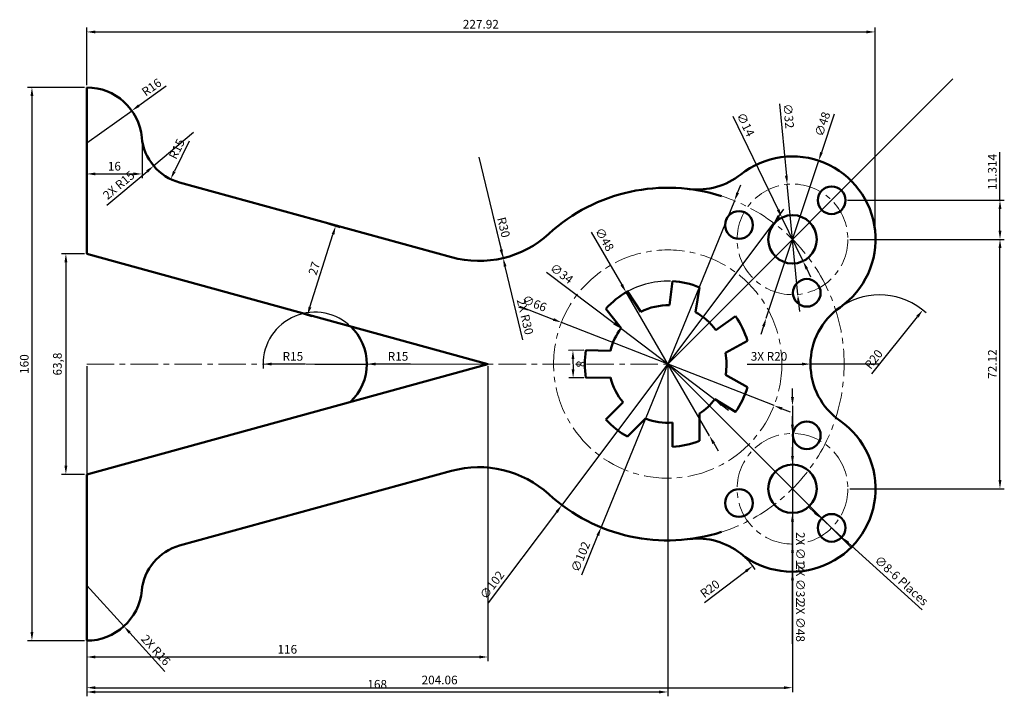
# Model space of a CAD drawing. Units: millimetres. Extents: x 1894 to 2178, y 716 to 912.
import ezdxf

# ---------------------------------------------------------------- set-up
doc = ezdxf.new("R2010")
doc.units = ezdxf.units.MM
doc.linetypes.add('CENTER', pattern=[50.8, 31.75, -6.35, 6.35, -6.35])
for name, color, linetype, lineweight in [('M-CNTR', 4, 'CENTER', 18), ('M-CONS', 8, 'Continuous', 13), ('M-DIMS', 2, 'Continuous', 25), ('M-OUTL', 7, 'Continuous', 50)]:
    doc.layers.add(name, color=color, linetype=linetype, lineweight=lineweight)
doc.styles.get("Standard").update_dxf_attribs({"font": 'arial.ttf'})
doc.dimstyles.new('ISO-25', dxfattribs={"dimtxt": 2.5, "dimasz": 2.5, "dimexe": 1.25, "dimexo": 0.625, "dimtad": 1, "dimtxsty": 'Standard', "dimcen": 2.5, "dimadec": 0, "dimazin": 0, "dimtfac": 1, "dimtmove": 0, "dimatfit": 3, "dimfxl": 1, "dimarcsym": 0})

# ---------------------------------------------------------------- blocks, each defined once
blk = doc.blocks.new('*U1')
blk.add_circle((0, 0), 4)
blk = doc.blocks.new('*U2')
at = {"layer": 'M-OUTL', "color": 0, "linetype": 'ByBlock', "lineweight": -2, "transparency": 16777216}
blk.add_blockref('*U1', (2128.28, 859.35), dxfattribs=at)
for p, rotation in [((2101.51, 852.18), 120), ((2121.11, 832.58), 240)]:
    blk.add_blockref('*U1', p, dxfattribs=dict(at, rotation=rotation))
blk = doc.blocks.new('*U3')
blk.add_circle((0, 0), 4)
blk = doc.blocks.new('*U4')
at = {"layer": 'M-OUTL', "color": 0, "linetype": 'ByBlock', "lineweight": -2, "transparency": 16777216}
for p, rotation in [((2121.11, 791.37), 120), ((2101.51, 771.77), 239.9999999999999)]:
    blk.add_blockref('*U3', p, dxfattribs=dict(at, rotation=rotation))
blk.add_blockref('*U3', (2128.28, 764.6), dxfattribs=at)
blk = doc.blocks.new('*D5')
at = {"layer": 'Defpoints', "color": 0, "transparency": 16777216}
for p in [(1912.93, 891.97), (1897.08, 731.97), (1912.91, 731.97)]:
    blk.add_point(p, dxfattribs=at)
at = {"layer": 'M-DIMS', "color": 0, "lineweight": -2, "transparency": 16777216}
for p, q in [((1912.3, 891.97), (1895.83, 891.97)), ((1897.08, 889.47), (1897.08, 734.47)), ((1912.28, 731.97), (1895.83, 731.97))]:
    blk.add_line(p, q, dxfattribs=at)
at = {"layer": 'M-DIMS', "color": 0, "transparency": 16777216}
for points in [[(1896.66, 889.47), (1897.5, 889.47), (1897.08, 891.97)], [(1896.66, 734.47), (1897.5, 734.47), (1897.08, 731.97)]]:
    blk.add_solid(points, dxfattribs=at)
at = {"layer": 'M-DIMS', "color": 0, "transparency": 16777216, "insert": (1895.18, 811.97), "char_height": 2.5, "attachment_point": 5, "rotation": 90}
blk.add_mtext('160', dxfattribs=at)
blk = doc.blocks.new('*D6')
at = {"layer": 'Defpoints', "color": 0, "transparency": 16777216}
for p in [(1912.91, 843.87), (1906.89, 780.07), (1912.91, 780.07)]:
    blk.add_point(p, dxfattribs=at)
at = {"layer": 'M-DIMS', "color": 0, "lineweight": -2, "transparency": 16777216}
for p, q in [((1912.28, 843.87), (1905.64, 843.87)), ((1906.89, 841.37), (1906.89, 782.57)), ((1912.28, 780.07), (1905.64, 780.07))]:
    blk.add_line(p, q, dxfattribs=at)
at = {"layer": 'M-DIMS', "color": 0, "transparency": 16777216}
for points in [[(1906.48, 841.37), (1907.31, 841.37), (1906.89, 843.87)], [(1906.48, 782.57), (1907.31, 782.57), (1906.89, 780.07)]]:
    blk.add_solid(points, dxfattribs=at)
at = {"layer": 'M-DIMS', "color": 0, "transparency": 16777216, "insert": (1904.76, 811.97), "char_height": 2.5, "attachment_point": 5, "rotation": 90}
blk.add_mtext('63,8', dxfattribs=at)
blk = doc.blocks.new('*D7')
at = {"layer": 'Defpoints', "color": 0, "transparency": 16777216}
for p in [(1912.91, 875.97), (1928.91, 875.97), (1928.91, 866.96)]:
    blk.add_point(p, dxfattribs=at)
at = {"layer": 'M-DIMS', "color": 0, "lineweight": -2, "transparency": 16777216}
for p, q in [((1912.91, 875.35), (1912.91, 865.71)), ((1928.91, 875.35), (1928.91, 865.71)), ((1915.41, 866.96), (1926.41, 866.96))]:
    blk.add_line(p, q, dxfattribs=at)
at = {"layer": 'M-DIMS', "color": 0, "transparency": 16777216}
for points in [[(1915.41, 867.38), (1915.41, 866.55), (1912.91, 866.96)], [(1926.41, 867.38), (1926.41, 866.55), (1928.91, 866.96)]]:
    blk.add_solid(points, dxfattribs=at)
at = {"layer": 'M-DIMS', "color": 0, "transparency": 16777216, "insert": (1920.91, 868.87), "char_height": 2.5, "attachment_point": 5}
blk.add_mtext('16', dxfattribs=at)
blk = doc.blocks.new('*D8')
at = {"layer": 'Defpoints', "color": 0, "transparency": 16777216}
for p in [(1979.07, 853.68), (1984.88, 851.84), (1970.91, 827.92)]:
    blk.add_point(p, dxfattribs=at)
at = {"layer": 'M-DIMS', "color": 0, "lineweight": -2, "transparency": 16777216}
for p, q in [((1979.67, 853.49), (1986.07, 851.46)), ((1977.47, 828.47), (1984.12, 849.46)), ((1971.5, 827.73), (1977.9, 825.71))]:
    blk.add_line(p, q, dxfattribs=at)
at = {"layer": 'M-DIMS', "color": 0, "transparency": 16777216}
for points in [[(1983.72, 849.58), (1984.52, 849.33), (1984.88, 851.84)], [(1977.07, 828.59), (1977.87, 828.34), (1976.71, 826.08)]]:
    blk.add_solid(points, dxfattribs=at)
at = {"layer": 'M-DIMS', "color": 0, "transparency": 16777216, "insert": (1979, 839.53), "char_height": 2.5, "attachment_point": 5, "rotation": 72.4174}
blk.add_mtext('27', dxfattribs=at)
blk = doc.blocks.new('*D9')
at = {"layer": 'Defpoints', "color": 0, "transparency": 16777216}
for p in [(1912.91, 811.97), (2028.91, 811.97), (2028.91, 727.25)]:
    blk.add_point(p, dxfattribs=at)
at = {"layer": 'M-DIMS', "color": 0, "lineweight": -2, "transparency": 16777216}
for p, q in [((1912.91, 811.35), (1912.91, 726)), ((2028.91, 811.35), (2028.91, 726)), ((1915.41, 727.25), (2026.41, 727.25))]:
    blk.add_line(p, q, dxfattribs=at)
at = {"layer": 'M-DIMS', "color": 0, "transparency": 16777216}
for points in [[(1915.41, 727.66), (1915.41, 726.83), (1912.91, 727.25)], [(2026.41, 727.66), (2026.41, 726.83), (2028.91, 727.25)]]:
    blk.add_solid(points, dxfattribs=at)
at = {"layer": 'M-DIMS', "color": 0, "transparency": 16777216, "insert": (1970.91, 729.15), "char_height": 2.5, "attachment_point": 5}
blk.add_mtext('116', dxfattribs=at)
blk = doc.blocks.new('*D10')
at = {"layer": 'Defpoints', "color": 0, "transparency": 16777216}
for p in [(2080.91, 811.97), (1912.91, 731.97), (2080.91, 717.13)]:
    blk.add_point(p, dxfattribs=at)
at = {"layer": 'M-DIMS', "color": 0, "lineweight": -2, "transparency": 16777216}
for p, q in [((2080.91, 811.35), (2080.91, 715.88)), ((1912.91, 731.35), (1912.91, 715.88)), ((1915.41, 717.13), (2078.41, 717.13))]:
    blk.add_line(p, q, dxfattribs=at)
at = {"layer": 'M-DIMS', "color": 0, "transparency": 16777216}
for points in [[(1915.41, 717.54), (1915.41, 716.71), (1912.91, 717.13)], [(2078.41, 717.54), (2078.41, 716.71), (2080.91, 717.13)]]:
    blk.add_solid(points, dxfattribs=at)
at = {"layer": 'M-DIMS', "color": 0, "transparency": 16777216, "insert": (1996.91, 719.03), "char_height": 2.5, "attachment_point": 5}
blk.add_mtext('168', dxfattribs=at)
blk = doc.blocks.new('*D11')
at = {"layer": 'Defpoints', "color": 0, "transparency": 16777216}
for p in [(2057.24, 815.96), (2053.55, 807.96), (2057.31, 807.99)]:
    blk.add_point(p, dxfattribs=at)
at = {"layer": 'M-DIMS', "color": 0, "lineweight": -2, "transparency": 16777216}
for p, q in [((2056.62, 815.95), (2052.24, 815.92)), ((2053.51, 813.43), (2053.53, 810.46)), ((2056.68, 807.98), (2052.3, 807.95))]:
    blk.add_line(p, q, dxfattribs=at)
at = {"layer": 'M-DIMS', "color": 0, "transparency": 16777216}
for points in [[(2053.92, 813.43), (2053.09, 813.42), (2053.49, 815.93)], [(2053.95, 810.46), (2053.12, 810.45), (2053.55, 807.96)]]:
    blk.add_solid(points, dxfattribs=at)
at = {"layer": 'M-DIMS', "color": 0, "transparency": 16777216, "insert": (2055.42, 811.96), "char_height": 2.5, "attachment_point": 5, "rotation": 270.4709}
blk.add_mtext('8', dxfattribs=at)
blk = doc.blocks.new('*D12')
at = {"layer": 'Defpoints', "color": 0, "transparency": 16777216}
for p in [(1963.91, 811.97), (1978.91, 811.97)]:
    blk.add_point(p, dxfattribs=at)
at = {"layer": 'M-DIMS', "color": 0, "lineweight": -2, "transparency": 16777216}
blk.add_line((1976.15, 811.97), (1966.41, 811.97), dxfattribs=at)
blk.add_arc((1978.91, 811.97), 15, 49.122, 184.7746, dxfattribs=at)
at = {"layer": 'M-DIMS', "color": 0, "transparency": 16777216}
blk.add_solid([(1966.41, 812.39), (1966.41, 811.56), (1963.91, 811.97)], dxfattribs=at)
at = {"layer": 'M-DIMS', "color": 0, "transparency": 16777216, "insert": (1972.53, 813.87), "char_height": 2.5, "attachment_point": 5}
blk.add_mtext('R15', dxfattribs=at)
blk = doc.blocks.new('*D13')
at = {"layer": 'Defpoints', "color": 0, "transparency": 16777216}
for p in [(1943.76, 878.95), (1937.18, 865.47)]:
    blk.add_point(p, dxfattribs=at)
at = {"layer": 'M-DIMS', "color": 0, "lineweight": -2, "transparency": 16777216}
blk.add_line((1942.55, 876.47), (1938.28, 867.72), dxfattribs=at)
at = {"layer": 'M-DIMS', "color": 0, "transparency": 16777216}
blk.add_solid([(1937.9, 867.9), (1938.65, 867.53), (1937.18, 865.47)], dxfattribs=at)
at = {"layer": 'M-DIMS', "color": 0, "transparency": 16777216, "insert": (1939.26, 874.05), "char_height": 2.5, "attachment_point": 5, "rotation": 63.9559}
blk.add_mtext('R15', dxfattribs=at)
blk = doc.blocks.new('*D14')
at = {"layer": 'Defpoints', "color": 0, "transparency": 16777216}
for p in [(1925.95, 885.25), (1912.91, 875.97)]:
    blk.add_point(p, dxfattribs=at)
at = {"layer": 'M-DIMS', "color": 0, "lineweight": -2, "transparency": 16777216}
for p, q in [((1935.91, 892.33), (1927.98, 886.69)), ((1912.91, 875.97), (1925.95, 885.25))]:
    blk.add_line(p, q, dxfattribs=at)
at = {"layer": 'M-DIMS', "color": 0, "transparency": 16777216}
blk.add_solid([(1927.74, 887.03), (1928.23, 886.35), (1925.95, 885.25)], dxfattribs=at)
at = {"layer": 'M-DIMS', "color": 0, "transparency": 16777216, "insert": (1931.86, 891.78), "char_height": 2.5, "attachment_point": 5, "rotation": 35.4167}
blk.add_mtext('R16', dxfattribs=at)
blk = doc.blocks.new('*D15')
at = {"layer": 'Defpoints', "color": 0, "transparency": 16777216}
for p in [(2026.31, 871.8), (2033.31, 842.63)]:
    blk.add_point(p, dxfattribs=at)
at = {"layer": 'M-DIMS', "color": 0, "lineweight": -2, "transparency": 16777216}
blk.add_line((2030.46, 854.51), (2032.73, 845.06), dxfattribs=at)
at = {"layer": 'M-DIMS', "color": 0, "transparency": 16777216}
blk.add_solid([(2033.13, 845.16), (2032.32, 844.97), (2033.31, 842.63)], dxfattribs=at)
at = {"layer": 'M-DIMS', "color": 0, "transparency": 16777216, "insert": (2033.15, 851.45), "char_height": 2.5, "attachment_point": 5, "rotation": 283.5033}
blk.add_mtext('R30', dxfattribs=at)
blk = doc.blocks.new('*D16')
at = {"layer": 'Defpoints', "color": 0, "transparency": 16777216}
for p in [(2105.49, 753.58), (2089.55, 741.5)]:
    blk.add_point(p, dxfattribs=at)
at = {"layer": 'M-DIMS', "color": 0, "lineweight": -2, "transparency": 16777216}
blk.add_line((2091.57, 743.03), (2103.5, 752.07), dxfattribs=at)
blk.add_arc((2089.55, 741.5), 20, 33.5739, 49.6574, dxfattribs=at)
at = {"layer": 'M-DIMS', "color": 0, "transparency": 16777216}
blk.add_solid([(2103.24, 752.4), (2103.75, 751.74), (2105.49, 753.58)], dxfattribs=at)
at = {"layer": 'M-DIMS', "color": 0, "transparency": 16777216, "insert": (2093.3, 746.73), "char_height": 2.5, "attachment_point": 5, "rotation": 37.1548}
blk.add_mtext('R20', dxfattribs=at)
blk = doc.blocks.new('*D17')
at = {"layer": 'Defpoints', "color": 0, "transparency": 16777216}
for p in [(2154.65, 827.61), (2142.18, 811.97)]:
    blk.add_point(p, dxfattribs=at)
at = {"layer": 'M-DIMS', "color": 0, "lineweight": -2, "transparency": 16777216}
blk.add_line((2139.93, 809.15), (2153.09, 825.65), dxfattribs=at)
blk.add_arc((2142.18, 811.97), 20, 47.8476, 123.1646, dxfattribs=at)
at = {"layer": 'M-DIMS', "color": 0, "transparency": 16777216}
blk.add_solid([(2152.76, 825.91), (2153.42, 825.4), (2154.65, 827.61)], dxfattribs=at)
at = {"layer": 'M-DIMS', "color": 0, "transparency": 16777216, "insert": (2140.69, 813.16), "char_height": 2.5, "attachment_point": 5, "rotation": 51.4286}
blk.add_mtext('R20', dxfattribs=at)
blk = doc.blocks.new('*D18')
at = {"layer": 'Defpoints', "color": 0, "transparency": 16777216}
for p in [(2113.92, 854.33), (2120.02, 841.74)]:
    blk.add_point(p, dxfattribs=at)
at = {"layer": 'M-DIMS', "color": 0, "lineweight": -2, "transparency": 16777216}
for p, q in [((2099.72, 883.62), (2112.83, 856.58)), ((2120.02, 841.74), (2113.92, 854.33)), ((2121.11, 839.49), (2122.2, 837.24))]:
    blk.add_line(p, q, dxfattribs=at)
at = {"layer": 'M-DIMS', "color": 0, "transparency": 16777216}
for points in [[(2113.2, 856.77), (2112.45, 856.4), (2113.92, 854.33)], [(2121.49, 839.67), (2120.74, 839.3), (2120.02, 841.74)]]:
    blk.add_solid(points, dxfattribs=at)
at = {"layer": 'M-DIMS', "color": 0, "transparency": 16777216, "insert": (2103.14, 881.09), "char_height": 2.5, "attachment_point": 5, "rotation": 295.8538}
blk.add_mtext('∅14', dxfattribs=at)
blk = doc.blocks.new('*D19')
at = {"layer": 'Defpoints', "color": 0, "transparency": 16777216}
for p in [(2115.45, 863.96), (2118.49, 832.11)]:
    blk.add_point(p, dxfattribs=at)
at = {"layer": 'M-DIMS', "color": 0, "lineweight": -2, "transparency": 16777216}
for p, q in [((2113.22, 887.23), (2115.21, 866.45)), ((2118.49, 832.11), (2115.45, 863.96)), ((2118.73, 829.62), (2118.97, 827.13))]:
    blk.add_line(p, q, dxfattribs=at)
at = {"layer": 'M-DIMS', "color": 0, "transparency": 16777216}
for points in [[(2115.62, 866.49), (2114.79, 866.41), (2115.45, 863.96)], [(2119.15, 829.66), (2118.32, 829.58), (2118.49, 832.11)]]:
    blk.add_solid(points, dxfattribs=at)
at = {"layer": 'M-DIMS', "color": 0, "transparency": 16777216, "insert": (2115.54, 883.67), "char_height": 2.5, "attachment_point": 5, "rotation": 275.4624}
blk.add_mtext('∅32', dxfattribs=at)
blk = doc.blocks.new('*D20')
at = {"layer": 'Defpoints', "color": 0, "transparency": 16777216}
for p in [(2124.55, 870.81), (2109.39, 825.26)]:
    blk.add_point(p, dxfattribs=at)
at = {"layer": 'M-DIMS', "color": 0, "lineweight": -2, "transparency": 16777216}
for p, q in [((2129.02, 884.22), (2125.34, 873.18)), ((2109.39, 825.26), (2124.55, 870.81)), ((2108.6, 822.89), (2107.81, 820.52))]:
    blk.add_line(p, q, dxfattribs=at)
at = {"layer": 'M-DIMS', "color": 0, "transparency": 16777216}
for points in [[(2124.95, 873.31), (2125.74, 873.05), (2124.55, 870.81)], [(2108.2, 823.02), (2108.99, 822.76), (2109.39, 825.26)]]:
    blk.add_solid(points, dxfattribs=at)
at = {"layer": 'M-DIMS', "color": 0, "transparency": 16777216, "insert": (2125.96, 881.26), "char_height": 2.5, "attachment_point": 5, "rotation": 71.5817}
blk.add_mtext('∅48', dxfattribs=at)
blk = doc.blocks.new('*D21')
at = {"layer": 'Defpoints', "color": 0, "transparency": 16777216}
for p in [(2125.32, 767.28), (2131.25, 761.91)]:
    blk.add_point(p, dxfattribs=at)
at = {"layer": 'M-DIMS', "color": 0, "lineweight": -2, "transparency": 16777216}
for p, q in [((2123.47, 768.96), (2121.62, 770.64)), ((2125.32, 767.28), (2131.25, 761.91)), ((2154.44, 740.87), (2133.1, 760.23))]:
    blk.add_line(p, q, dxfattribs=at)
at = {"layer": 'M-DIMS', "color": 0, "transparency": 16777216}
for points in [[(2123.75, 769.27), (2123.19, 768.66), (2125.32, 767.28)], [(2133.38, 760.54), (2132.82, 759.92), (2131.25, 761.91)]]:
    blk.add_solid(points, dxfattribs=at)
at = {"layer": 'M-DIMS', "color": 0, "transparency": 16777216, "insert": (2148.28, 749.11), "char_height": 2.5, "attachment_point": 5, "rotation": 317.785}
blk.add_mtext('∅8-6 Places', dxfattribs=at)
blk = doc.blocks.new('*D22')
at = {"layer": 'Defpoints', "color": 0, "transparency": 16777216}
for p in [(2100.18, 859.19), (2061.64, 764.75)]:
    blk.add_point(p, dxfattribs=at)
at = {"layer": 'M-DIMS', "color": 0, "lineweight": -2, "transparency": 16777216}
for p, q in [((2101.12, 861.51), (2102.07, 863.82)), ((2100.18, 859.19), (2061.64, 764.75)), ((2056.02, 751), (2060.69, 762.44))]:
    blk.add_line(p, q, dxfattribs=at)
at = {"layer": 'M-DIMS', "color": 0, "transparency": 16777216}
for points in [[(2100.74, 861.66), (2101.51, 861.35), (2100.18, 859.19)], [(2060.31, 762.6), (2061.08, 762.28), (2061.64, 764.75)]]:
    blk.add_solid(points, dxfattribs=at)
at = {"layer": 'M-DIMS', "color": 0, "transparency": 16777216, "insert": (2055.99, 756.13), "char_height": 2.5, "attachment_point": 5, "rotation": 67.7998}
blk.add_mtext('∅102', dxfattribs=at)
blk = doc.blocks.new('*D23')
at = {"layer": 'Defpoints', "color": 0, "transparency": 16777216}
for p in [(2050.17, 823.99), (2111.64, 799.96)]:
    blk.add_point(p, dxfattribs=at)
at = {"layer": 'M-DIMS', "color": 0, "lineweight": -2, "transparency": 16777216}
for p, q in [((2038.01, 828.74), (2047.84, 824.9)), ((2111.64, 799.96), (2050.17, 823.99)), ((2113.97, 799.05), (2116.3, 798.14))]:
    blk.add_line(p, q, dxfattribs=at)
at = {"layer": 'M-DIMS', "color": 0, "transparency": 16777216}
for points in [[(2047.99, 825.28), (2047.69, 824.51), (2050.17, 823.99)], [(2114.12, 799.44), (2113.82, 798.66), (2111.64, 799.96)]]:
    blk.add_solid(points, dxfattribs=at)
at = {"layer": 'M-DIMS', "color": 0, "transparency": 16777216, "insert": (2042.25, 829.2), "char_height": 2.5, "attachment_point": 5, "rotation": 338.6521}
blk.add_mtext('∅66', dxfattribs=at)
blk = doc.blocks.new('*D24')
at = {"layer": 'Defpoints', "color": 0, "transparency": 16777216}
for p in [(2067.37, 822.25), (2094.45, 801.69)]:
    blk.add_point(p, dxfattribs=at)
at = {"layer": 'M-DIMS', "color": 0, "lineweight": -2, "transparency": 16777216}
for p, q in [((2045.85, 838.59), (2065.38, 823.77)), ((2094.45, 801.69), (2067.37, 822.25)), ((2096.44, 800.18), (2098.43, 798.67))]:
    blk.add_line(p, q, dxfattribs=at)
at = {"layer": 'M-DIMS', "color": 0, "transparency": 16777216}
for points in [[(2065.63, 824.1), (2065.13, 823.43), (2067.37, 822.25)], [(2096.69, 800.51), (2096.19, 799.85), (2094.45, 801.69)]]:
    blk.add_solid(points, dxfattribs=at)
at = {"layer": 'M-DIMS', "color": 0, "transparency": 16777216, "insert": (2050.05, 837.88), "char_height": 2.5, "attachment_point": 5, "rotation": 322.7886}
blk.add_mtext('∅34', dxfattribs=at)
blk = doc.blocks.new('*D25')
at = {"layer": 'Defpoints', "color": 0, "transparency": 16777216}
for p in [(2068.87, 832.73), (2092.95, 791.21)]:
    blk.add_point(p, dxfattribs=at)
at = {"layer": 'M-DIMS', "color": 0, "lineweight": -2, "transparency": 16777216}
for p, q in [((2058.77, 850.15), (2067.61, 834.9)), ((2092.95, 791.21), (2068.87, 832.73)), ((2094.2, 789.05), (2095.46, 786.89))]:
    blk.add_line(p, q, dxfattribs=at)
blk.add_arc((2080.91, 811.97), 24, 88.1953, 123.0942, dxfattribs=at)
at = {"layer": 'M-DIMS', "color": 0, "transparency": 16777216}
for points in [[(2067.97, 835.11), (2067.25, 834.69), (2068.87, 832.73)], [(2094.56, 789.26), (2093.84, 788.84), (2092.95, 791.21)]]:
    blk.add_solid(points, dxfattribs=at)
at = {"layer": 'M-DIMS', "color": 0, "transparency": 16777216, "insert": (2062.37, 847.87), "char_height": 2.5, "attachment_point": 5, "rotation": 300.11}
blk.add_mtext('∅48', dxfattribs=at)
blk = doc.blocks.new('*D26')
at = {"layer": 'Defpoints', "color": 0, "transparency": 16777216}
for p in [(2140.83, 908.03), (1912.91, 891.97), (2140.83, 850.61)]:
    blk.add_point(p, dxfattribs=at)
at = {"layer": 'M-DIMS', "color": 0, "lineweight": -2, "transparency": 16777216}
for p, q in [((1912.91, 892.6), (1912.91, 909.28)), ((2140.83, 851.23), (2140.83, 909.28)), ((1915.41, 908.03), (2138.33, 908.03))]:
    blk.add_line(p, q, dxfattribs=at)
at = {"layer": 'M-DIMS', "color": 0, "transparency": 16777216}
for points in [[(1915.41, 908.44), (1915.41, 907.61), (1912.91, 908.03)], [(2138.33, 908.44), (2138.33, 907.61), (2140.83, 908.03)]]:
    blk.add_solid(points, dxfattribs=at)
at = {"layer": 'M-DIMS', "color": 0, "transparency": 16777216, "insert": (2026.87, 909.93), "char_height": 2.5, "attachment_point": 5}
blk.add_mtext('227.92', dxfattribs=at)
blk = doc.blocks.new('*D27')
at = {"layer": 'Defpoints', "color": 0, "transparency": 16777216}
for p in [(2132.97, 848.04), (2176.96, 848.04), (2132.97, 775.91)]:
    blk.add_point(p, dxfattribs=at)
at = {"layer": 'M-DIMS', "color": 0, "lineweight": -2, "transparency": 16777216}
for p, q in [((2133.59, 848.04), (2178.21, 848.04)), ((2176.96, 778.41), (2176.96, 845.54)), ((2133.59, 775.91), (2178.21, 775.91))]:
    blk.add_line(p, q, dxfattribs=at)
at = {"layer": 'M-DIMS', "color": 0, "transparency": 16777216}
for points in [[(2176.55, 845.54), (2177.38, 845.54), (2176.96, 848.04)], [(2176.55, 778.41), (2177.38, 778.41), (2176.96, 775.91)]]:
    blk.add_solid(points, dxfattribs=at)
at = {"layer": 'M-DIMS', "color": 0, "transparency": 16777216, "insert": (2175.08, 811.97), "char_height": 2.5, "attachment_point": 5, "rotation": 90}
blk.add_mtext('72.12', dxfattribs=at)
blk = doc.blocks.new('*D28')
at = {"layer": 'Defpoints', "color": 0, "transparency": 16777216}
for p in [(2116.97, 759.91), (1912.91, 731.97), (2116.97, 718.37)]:
    blk.add_point(p, dxfattribs=at)
at = {"layer": 'M-DIMS', "color": 0, "lineweight": -2, "transparency": 16777216}
for p, q in [((2116.97, 759.29), (2116.97, 717.12)), ((1912.91, 731.35), (1912.91, 717.12)), ((1915.41, 718.37), (2114.47, 718.37))]:
    blk.add_line(p, q, dxfattribs=at)
at = {"layer": 'M-DIMS', "color": 0, "transparency": 16777216}
for points in [[(1915.41, 718.79), (1915.41, 717.96), (1912.91, 718.37)], [(2114.47, 718.79), (2114.47, 717.96), (2116.97, 718.37)]]:
    blk.add_solid(points, dxfattribs=at)
at = {"layer": 'M-DIMS', "color": 0, "transparency": 16777216, "insert": (2014.94, 720.27), "char_height": 2.5, "attachment_point": 5}
blk.add_mtext('204.06', dxfattribs=at)
blk = doc.blocks.new('*D29')
at = {"layer": 'Defpoints', "color": 0, "transparency": 16777216}
for p in [(2132.28, 859.35), (2176.96, 859.35), (2132.97, 848.04)]:
    blk.add_point(p, dxfattribs=at)
at = {"layer": 'M-DIMS', "color": 0, "lineweight": -2, "transparency": 16777216}
for p, q in [((2176.96, 859.35), (2176.96, 873.23)), ((2132.91, 859.35), (2178.21, 859.35)), ((2176.96, 850.54), (2176.96, 856.85)), ((2133.59, 848.04), (2178.21, 848.04))]:
    blk.add_line(p, q, dxfattribs=at)
at = {"layer": 'M-DIMS', "color": 0, "transparency": 16777216}
for points in [[(2176.55, 856.85), (2177.38, 856.85), (2176.96, 859.35)], [(2176.55, 850.54), (2177.38, 850.54), (2176.96, 848.04)]]:
    blk.add_solid(points, dxfattribs=at)
at = {"layer": 'M-DIMS', "color": 0, "transparency": 16777216, "insert": (2175.06, 867.54), "char_height": 2.5, "attachment_point": 5, "rotation": 90}
blk.add_mtext('11.314', dxfattribs=at)
blk = doc.blocks.new('*D30')
at = {"layer": 'Defpoints', "color": 0, "transparency": 16777216}
for p in [(1912.91, 747.97), (1923.66, 736.13)]:
    blk.add_point(p, dxfattribs=at)
at = {"layer": 'M-DIMS', "color": 0, "lineweight": -2, "transparency": 16777216}
for p, q in [((1912.91, 747.97), (1923.66, 736.13)), ((1935.52, 723.07), (1925.35, 734.28))]:
    blk.add_line(p, q, dxfattribs=at)
at = {"layer": 'M-DIMS', "color": 0, "transparency": 16777216}
blk.add_solid([(1925.65, 734.56), (1925.04, 734), (1923.66, 736.13)], dxfattribs=at)
at = {"layer": 'M-DIMS', "color": 0, "transparency": 16777216, "insert": (1932.68, 729.03), "char_height": 2.5, "attachment_point": 5, "rotation": 312.2494}
blk.add_mtext('2X R16', dxfattribs=at)
blk = doc.blocks.new('*D31')
at = {"layer": 'Defpoints', "color": 0, "transparency": 16777216}
for p in [(1943.76, 878.95), (1932.28, 869.29)]:
    blk.add_point(p, dxfattribs=at)
at = {"layer": 'M-DIMS', "color": 0, "lineweight": -2, "transparency": 16777216}
for p, q in [((1943.76, 878.95), (1932.28, 869.29)), ((1918.77, 857.93), (1930.37, 867.68))]:
    blk.add_line(p, q, dxfattribs=at)
at = {"layer": 'M-DIMS', "color": 0, "transparency": 16777216}
blk.add_solid([(1930.1, 868), (1930.64, 867.36), (1932.28, 869.29)], dxfattribs=at)
at = {"layer": 'M-DIMS', "color": 0, "transparency": 16777216, "insert": (1922.39, 863.46), "char_height": 2.5, "attachment_point": 5, "rotation": 40.0622}
blk.add_mtext('2X R15', dxfattribs=at)
blk = doc.blocks.new('*D32')
at = {"layer": 'Defpoints', "color": 0, "transparency": 16777216}
for p in [(1978.91, 811.97), (1993.91, 811.97)]:
    blk.add_point(p, dxfattribs=at)
at = {"layer": 'M-DIMS', "color": 0, "lineweight": -2, "transparency": 16777216}
for p, q in [((1978.91, 811.97), (1993.91, 811.97)), ((2006.53, 811.97), (1996.41, 811.97))]:
    blk.add_line(p, q, dxfattribs=at)
at = {"layer": 'M-DIMS', "color": 0, "transparency": 16777216}
blk.add_solid([(1996.41, 812.39), (1996.41, 811.56), (1993.91, 811.97)], dxfattribs=at)
at = {"layer": 'M-DIMS', "color": 0, "transparency": 16777216, "insert": (2002.91, 813.87), "char_height": 2.5, "attachment_point": 5, "rotation": 0.0009}
blk.add_mtext('R15', dxfattribs=at)
blk = doc.blocks.new('*D33')
at = {"layer": 'Defpoints', "color": 0, "transparency": 16777216}
for p in [(2026.31, 871.8), (2033.31, 842.63)]:
    blk.add_point(p, dxfattribs=at)
at = {"layer": 'M-DIMS', "color": 0, "lineweight": -2, "transparency": 16777216}
for p, q in [((2026.31, 871.8), (2033.31, 842.63)), ((2038.99, 818.99), (2033.9, 840.2))]:
    blk.add_line(p, q, dxfattribs=at)
at = {"layer": 'M-DIMS', "color": 0, "transparency": 16777216}
blk.add_solid([(2034.3, 840.3), (2033.49, 840.11), (2033.31, 842.63)], dxfattribs=at)
at = {"layer": 'M-DIMS', "color": 0, "transparency": 16777216, "insert": (2039.36, 825.58), "char_height": 2.5, "attachment_point": 5, "rotation": 283.5041}
blk.add_mtext('2X R30', dxfattribs=at)
blk = doc.blocks.new('*D34')
at = {"layer": 'Defpoints', "color": 0, "transparency": 16777216}
for p in [(2111.51, 852.77), (2050.3, 771.18)]:
    blk.add_point(p, dxfattribs=at)
at = {"layer": 'M-DIMS', "color": 0, "lineweight": -2, "transparency": 16777216}
for p, q in [((2113.01, 854.77), (2114.51, 856.77)), ((2111.51, 852.77), (2050.3, 771.18)), ((2029.1, 742.91), (2048.8, 769.18))]:
    blk.add_line(p, q, dxfattribs=at)
at = {"layer": 'M-DIMS', "color": 0, "transparency": 16777216}
for points in [[(2112.68, 855.02), (2113.34, 854.52), (2111.51, 852.77)], [(2048.47, 769.43), (2049.14, 768.93), (2050.3, 771.18)]]:
    blk.add_solid(points, dxfattribs=at)
at = {"layer": 'M-DIMS', "color": 0, "transparency": 16777216, "insert": (2030.36, 747.88), "char_height": 2.5, "attachment_point": 5, "rotation": 53.1256}
blk.add_mtext('∅102', dxfattribs=at)
blk = doc.blocks.new('*D35')
at = {"layer": 'Defpoints', "color": 0, "transparency": 16777216}
for p in [(2122.18, 811.97), (2142.18, 811.97)]:
    blk.add_point(p, dxfattribs=at)
at = {"layer": 'M-DIMS', "color": 0, "lineweight": -2, "transparency": 16777216}
for p, q in [((2103.89, 811.97), (2119.68, 811.97)), ((2142.18, 811.97), (2122.18, 811.97))]:
    blk.add_line(p, q, dxfattribs=at)
at = {"layer": 'M-DIMS', "color": 0, "transparency": 16777216}
blk.add_solid([(2119.68, 812.39), (2119.68, 811.55), (2122.18, 811.97)], dxfattribs=at)
at = {"layer": 'M-DIMS', "color": 0, "transparency": 16777216, "insert": (2110.18, 813.87), "char_height": 2.5, "attachment_point": 5, "rotation": 0.0079}
blk.add_mtext('3X R20', dxfattribs=at)
blk = doc.blocks.new('*D36')
at = {"layer": 'Defpoints', "color": 0, "transparency": 16777216}
for p in [(2116.97, 799.91), (2116.97, 751.91)]:
    blk.add_point(p, dxfattribs=at)
at = {"layer": 'M-DIMS', "color": 0, "lineweight": -2, "transparency": 16777216}
for p, q in [((2116.97, 802.41), (2116.97, 804.91)), ((2116.97, 799.91), (2116.97, 751.91)), ((2116.97, 731.09), (2116.97, 749.41))]:
    blk.add_line(p, q, dxfattribs=at)
at = {"layer": 'M-DIMS', "color": 0, "transparency": 16777216}
for points in [[(2117.39, 802.41), (2116.55, 802.41), (2116.97, 799.91)], [(2117.39, 749.41), (2116.55, 749.41), (2116.97, 751.91)]]:
    blk.add_solid(points, dxfattribs=at)
at = {"layer": 'M-DIMS', "color": 0, "transparency": 16777216, "insert": (2118.94, 737.51), "char_height": 2.5, "attachment_point": 5, "rotation": 270.0011}
blk.add_mtext('2X ∅48', dxfattribs=at)
blk = doc.blocks.new('*D37')
at = {"layer": 'Defpoints', "color": 0, "transparency": 16777216}
for p in [(2116.97, 791.91), (2116.97, 759.91)]:
    blk.add_point(p, dxfattribs=at)
at = {"layer": 'M-DIMS', "color": 0, "lineweight": -2, "transparency": 16777216}
for p, q in [((2116.97, 794.41), (2116.97, 796.91)), ((2116.97, 791.91), (2116.97, 759.91)), ((2116.97, 742.1), (2116.97, 757.41))]:
    blk.add_line(p, q, dxfattribs=at)
at = {"layer": 'M-DIMS', "color": 0, "transparency": 16777216}
for points in [[(2117.39, 794.41), (2116.55, 794.41), (2116.97, 791.91)], [(2117.39, 757.41), (2116.55, 757.41), (2116.97, 759.91)]]:
    blk.add_solid(points, dxfattribs=at)
at = {"layer": 'M-DIMS', "color": 0, "transparency": 16777216, "insert": (2118.94, 748.51), "char_height": 2.5, "attachment_point": 5, "rotation": 270.0017}
blk.add_mtext('2X ∅32', dxfattribs=at)
blk = doc.blocks.new('*D38')
at = {"layer": 'Defpoints', "color": 0, "transparency": 16777216}
for p in [(2116.97, 782.91), (2116.97, 768.91)]:
    blk.add_point(p, dxfattribs=at)
at = {"layer": 'M-DIMS', "color": 0, "lineweight": -2, "transparency": 16777216}
for p, q in [((2116.97, 785.41), (2116.97, 787.91)), ((2116.97, 782.91), (2116.97, 768.91)), ((2116.97, 751.09), (2116.97, 766.41))]:
    blk.add_line(p, q, dxfattribs=at)
at = {"layer": 'M-DIMS', "color": 0, "transparency": 16777216}
for points in [[(2117.39, 785.41), (2116.55, 785.41), (2116.97, 782.91)], [(2117.39, 766.41), (2116.55, 766.41), (2116.97, 768.91)]]:
    blk.add_solid(points, dxfattribs=at)
at = {"layer": 'M-DIMS', "color": 0, "transparency": 16777216, "insert": (2118.94, 757.5), "char_height": 2.5, "attachment_point": 5, "rotation": 270.0037}
blk.add_mtext('2X ∅14', dxfattribs=at)

msp = doc.modelspace()

# ---------------------------------------------------------------- linework, layer by layer
at = {"layer": 'M-CNTR', "ltscale": 0.25}
for p, q in [((1912.9071, 811.9728), (2028.9071, 811.9728)), ((1993.9071, 811.9728), (2080.9071, 811.9728))]:
    msp.add_line(p, q, dxfattribs=at)
for centre, radius in [((2116.9695, 848.0352), 16), ((2080.9071, 811.9728), 33), ((2116.9695, 775.9103), 16)]:
    msp.add_circle(centre, radius, dxfattribs=at)
msp.add_arc((2080.9071, 811.9728), 51, 227.617124, 132.382876, dxfattribs=at)
at = {"layer": 'M-CONS'}
for p, q in [((2080.9071, 811.9728), (2163.3627, 894.4283)), ((1912.9071, 891.9728), (1912.9071, 875.9728)), ((1928.9071, 874.9728), (1928.9071, 875.9728)), ((2080.9071, 811.9728), (2133.9401, 758.9398))]:
    msp.add_line(p, q, dxfattribs=at)
at = {"layer": 'M-OUTL'}
for p, q in [((1912.9071, 843.8728), (1912.9071, 891.9728)), ((1939.7868, 864.4832), (2018.3518, 842.8778)), ((1912.9071, 843.8728), (2028.9071, 811.9728)), ((2082.2873, 835.9331), (2081.404, 828.9655)), ((2090.0596, 834.1591), (2088.9195, 826.9662)), ((2069.2676, 832.9614), (2069.2676, 832.9614)), ((2069.2676, 832.9614), (2073.167, 827.1085)), ((2063.0347, 827.9908), (2067.4235, 822.3262)), ((2100.5005, 825.8327), (2094.7858, 821.7902)), ((2103.9595, 818.65), (2097.5958, 815.211)), ((2057.2404, 815.9589), (2064.3462, 815.8116)), ((1912.9071, 780.0728), (2028.9071, 811.9728)), ((2103.9595, 805.2955), (2097.6201, 808.8624)), ((2057.2404, 807.9867), (2064.367, 808.0453)), ((2063.0347, 795.9547), (2067.9949, 800.9149)), ((2100.5005, 798.1128), (2094.5398, 801.8165)), ((2090.0596, 789.7865), (2090.0596, 797.6468)), ((2069.2676, 790.9841), (2074.507, 796.2235)), ((2082.2873, 788.0125), (2082.2873, 795.0289)), ((1912.9071, 731.9728), (1912.9071, 780.0728)), ((1939.7868, 759.4624), (2018.3518, 781.0677))]:
    msp.add_line(p, q, dxfattribs=at)
for centre in [(2116.9695, 848.0352), (2116.9695, 775.9103)]:
    msp.add_circle(centre, 7, dxfattribs=at)
for centre, radius, start, end in [((1912.9071, 875.9728), 16, 5.504221, 90), ((1943.7642, 878.9463), 15, 185.504221, 254.623749), ((2116.9695, 848.0352), 24, 304.955114, 128.552109), ((2089.5476, 882.445), 20, 263.009939, 308.552109), ((2080.9071, 811.9728), 51, 72.217917, 132.382876), ((2026.3065, 871.804), 30, 254.623749, 312.382876), ((2086.2476, 835.371), 4, 171.923049, 173.627946), ((2080.9071, 811.9728), 24, 67.582473, 86.703241), ((2080.9071, 811.9728), 24, 119.011045, 138.131812), ((2065.9433, 830.7367), 4, 33.554237, 33.791237), ((2080.9071, 811.9728), 17, 88.324877, 117.084273), ((2080.9071, 811.9728), 17, 35.274669, 61.880301), ((2102.5303, 822.386), 4, 120.494478, 130.054861), ((2080.9071, 811.9728), 24, 16.153902, 35.274669), ((2142.1787, 811.9728), 20, 124.955114, 235.044873), ((1978.9071, 811.9728), 15, 313.265313, 46.734687), ((2080.9071, 811.9728), 17, 142.481011, 166.949123), ((2080.9071, 811.9728), 24, 170.439616, 189.560384), ((2080.9071, 811.9728), 17, 349.457452, 10.981096), ((2080.9071, 811.9728), 17, 193.357728, 220.576426), ((2080.9071, 811.9728), 24, 324.725331, 343.846098), ((2080.9071, 811.9728), 17, 302.573491, 323.314238), ((2102.5303, 801.5596), 4, 236.785144, 239.505522), ((2065.9433, 793.2088), 4, 133.35162, 136.64838), ((2080.9071, 811.9728), 24, 221.868188, 240.988955), ((2080.9071, 811.9728), 17, 247.884422, 274.656806), ((2116.9695, 775.9103), 24, 231.447878, 55.044873), ((2086.2476, 788.5745), 4, 171.923049, 188.076951), ((2080.9071, 811.9728), 24, 273.296759, 292.417527), ((2026.3065, 752.1416), 30, 47.617124, 105.376251), ((2080.9071, 811.9728), 51, 227.617124, 287.78207), ((2089.5476, 741.5005), 20, 51.447878, 96.990048), ((1943.7642, 744.9993), 15, 105.376251, 174.495779), ((1912.9071, 747.9728), 16, 270, 354.495779)]:
    msp.add_arc(centre, radius, start, end, dxfattribs=at)

# ---------------------------------------------------------------- block references
for name in ['*U2', '*U4']:
    msp.add_blockref(name, (0, 0), dxfattribs=at)

# ---------------------------------------------------------------- dimensions: what is measured, and where the dimension line sits
at = {"layer": 'M-DIMS'}
for base, p1, p2, override, picture, middle in [((2140.8312, 908.0283), (1912.9071, 891.9728), (2140.8312, 850.6081), {"dimdec": 2, "dimlfac": 1, "dimrnd": 0, "dimzin": 0, "dimdsep": 46, "dimlunit": 2}, '*D26', (2026.8692, 909.9298)), ((1928.9071, 866.9642), (1912.9071, 875.9728), (1928.9071, 875.9728), {"dimclrd": 0, "dimclre": 0, "dimclrt": 0}, '*D7', (1920.9071, 868.8656)), ((2028.9071, 727.2466), (1912.9071, 811.9728), (2028.9071, 811.9728), {"dimclrd": 0, "dimclre": 0, "dimclrt": 0}, '*D9', (1970.9071, 729.1481)), ((2080.9071, 717.1271), (1912.9071, 731.9728), (2080.9071, 811.9728), {"dimclrd": 0, "dimclre": 0, "dimclrt": 0}, '*D10', (1996.9071, 719.0285)), ((2116.9695, 718.3728), (1912.9071, 731.9728), (2116.9695, 759.9103), {"dimdec": 2, "dimlfac": 1, "dimrnd": 0, "dimzin": 0, "dimdsep": 46, "dimlunit": 2}, '*D28', (2014.9383, 720.2742))]:
    dim = msp.add_linear_dim(base=base, p1=p1, p2=p2, dimstyle='ISO-25', override=override, dxfattribs=at)
    dim.commit()
    dim.dimension.update_dxf_attribs({"geometry": picture, "text_midpoint": middle})
dim = msp.add_radius_dim(center=(1912.9071, 875.9728), mpoint=(1925.9464, 885.2451), dimstyle='ISO-25', override={"dimclrd": 0, "dimclre": 0, "dimclrt": 0}, dxfattribs=at)
dim.commit()
dim.dimension.update_dxf_attribs({"geometry": '*D14', "text_midpoint": (1931.8622, 891.7849)})
for base, p1, p2, override, picture, middle in [((1897.0791, 731.9728), (1912.9274, 891.9728), (1912.9071, 731.9728), {"dimclrd": 0, "dimclre": 0, "dimclrt": 0}, '*D5', (1895.1776, 811.9728)), ((2176.9627, 859.3489), (2132.9695, 848.0352), (2132.2832, 859.3489), {"dimdec": 3, "dimlfac": 1, "dimrnd": 0, "dimzin": 0, "dimdsep": 46, "dimlunit": 2}, '*D29', (2175.0604, 867.5404)), ((2176.9627, 848.0352), (2132.9695, 775.9103), (2132.9695, 848.0352), {"dimdec": 2, "dimlfac": 1, "dimrnd": 0, "dimzin": 0, "dimdsep": 46, "dimlunit": 2}, '*D27', (2175.0825, 811.9728)), ((1906.8923, 780.0728), (1912.9071, 843.8728), (1912.9071, 780.0728), {"dimclrd": 0, "dimclre": 0, "dimclrt": 0}, '*D6', (1904.7649, 811.9728))]:
    dim = msp.add_linear_dim(base=base, p1=p1, p2=p2, angle=90, dimstyle='ISO-25', override=override, dxfattribs=at)
    dim.commit()
    dim.dimension.update_dxf_attribs({"geometry": picture, "text_midpoint": middle})
for p1, p2, override, picture, middle in [((2118.4926, 832.1079), (2115.4465, 863.9626), {"dimclrd": 0, "dimclre": 0, "dimclrt": 0}, '*D19', (2113.5796, 883.4853)), ((2120.0221, 841.7358), (2113.917, 854.3346), {"dimclrd": 0, "dimclre": 0, "dimclrt": 0}, '*D18', (2101.3677, 880.2318)), ((2109.3867, 825.2646), (2124.5524, 870.8058), {"dimclrd": 0, "dimclre": 0, "dimclrt": 0}, '*D20', (2127.8268, 880.6385)), ((2100.1771, 859.1921), (2061.6371, 764.7534), {"dimclrd": 0, "dimclre": 0, "dimclrt": 0}, '*D22', (2057.8121, 755.3808)), ((2111.5103, 852.7704), (2050.3039, 771.1752), {"dimdec": 0, "dimlfac": 1, "dimrnd": 0, "dimzin": 0, "dimdsep": 46, "dimlunit": 2}, '*D34', (2031.942, 746.6966)), ((2092.947, 791.2112), (2068.8672, 832.7343), {"dimclrd": 0, "dimclre": 0, "dimclrt": 0}, '*D25', (2060.6616, 846.884)), ((2094.4461, 801.6919), (2067.3681, 822.2536), {"dimclrd": 0, "dimclre": 0, "dimclrt": 0}, '*D24', (2048.8568, 836.3103)), ((2111.6429, 799.9598), (2050.1713, 823.9858), {"dimclrd": 0, "dimclre": 0, "dimclrt": 0}, '*D23', (2041.5297, 827.3633))]:
    dim = msp.add_diameter_dim_2p(p1=p1, p2=p2, dimstyle='ISO-25', override=override, dxfattribs=at)
    dim.commit()
    dim.dimension.update_dxf_attribs({"geometry": picture, "text_midpoint": middle, "dimtype": 163})
for center, mpoint, picture, middle in [((1943.7642, 878.9463), (1932.284, 869.292), '*D31', (1922.39, 863.456)), ((1912.9071, 747.9728), (1923.6648, 736.1292), '*D30', (1932.6822, 729.0296))]:
    dim = msp.add_radius_dim(center=center, mpoint=mpoint, text='2X <>', dimstyle='ISO-25', override={"dimdec": 0, "dimlfac": 1, "dimrnd": 0, "dimzin": 0, "dimdsep": 46, "dimlunit": 2}, dxfattribs=at)
    dim.commit()
    dim.dimension.update_dxf_attribs({"geometry": picture, "text_midpoint": middle})
for center, mpoint, override, picture, middle in [((1943.7642, 878.9463), (1937.1782, 865.4694), {"dimclrd": 0, "dimclre": 0, "dimclrt": 0}, '*D13', (1940.9635, 873.2152)), ((2026.3065, 871.804), (2033.3115, 842.6333), {"dimclrd": 0, "dimclre": 0, "dimclrt": 0}, '*D15', (2031.3016, 851.0029)), ((2142.1787, 811.9728), (2154.6485, 827.6094), {"dimclrd": 0, "dimclre": 0, "dimclrt": 0}, '*D17', (2142.1787, 811.9728)), ((1978.9071, 811.9728), (1963.9071, 811.9728), {"dimclrd": 0, "dimclre": 0, "dimclrt": 0}, '*D12', (1972.5283, 811.9728)), ((1978.9071, 811.9728), (1993.9071, 811.973), {"dimdec": 0, "dimlfac": 1, "dimrnd": 0, "dimzin": 0, "dimdsep": 46, "dimlunit": 2}, '*D32', (2002.9071, 811.9731)), ((2089.5476, 741.5005), (2105.4877, 753.5799), {"dimclrd": 0, "dimclre": 0, "dimclrt": 0}, '*D16', (2094.4477, 745.2138))]:
    dim = msp.add_radius_dim(center=center, mpoint=mpoint, dimstyle='ISO-25', override=override, dxfattribs=at)
    dim.commit()
    dim.dimension.update_dxf_attribs({"geometry": picture, "text_midpoint": middle, "dimtype": 164})
for center, mpoint, text, picture, middle in [((2026.3065, 871.804), (2033.3119, 842.6334), '2X <>', '*D33', (2037.5152, 825.131)), ((2142.1787, 811.9728), (2122.1787, 811.97), '3X <>', '*D35', (2110.1787, 811.9683))]:
    dim = msp.add_radius_dim(center=center, mpoint=mpoint, text=text, dimstyle='ISO-25', override={"dimdec": 0, "dimlfac": 1, "dimrnd": 0, "dimzin": 0, "dimdsep": 46, "dimlunit": 2}, dxfattribs=at)
    dim.commit()
    dim.dimension.update_dxf_attribs({"geometry": picture, "text_midpoint": middle, "dimtype": 164})
for p1, p2, distance, picture, middle in [((1970.9071, 827.9228), (1979.0693, 853.6805), -6.0905, '*D8', (1979.0019, 839.5298)), ((2057.2404, 815.9589), (2057.3059, 807.9872), -3.753, '*D11', (2055.4217, 811.9578))]:
    dim = msp.add_aligned_dim(p1=p1, p2=p2, distance=distance, dimstyle='ISO-25', override={"dimdec": 0, "dimclrd": 0, "dimclre": 0, "dimclrt": 0}, dxfattribs=at)
    dim.commit()
    dim.dimension.update_dxf_attribs({"geometry": picture, "text_midpoint": middle})
for p1, p2, text, override, picture, middle in [((2116.9691, 799.9103), (2116.97, 751.9103), '2X <>', {"dimdec": 0, "dimlfac": 1, "dimrnd": 0, "dimzin": 0, "dimdsep": 46, "dimlunit": 2}, '*D36', (2116.9703, 737.5103)), ((2116.9691, 791.9103), (2116.97, 759.9103), '2X <>', {"dimdec": 0, "dimlfac": 1, "dimrnd": 0, "dimzin": 0, "dimdsep": 46, "dimlunit": 2}, '*D37', (2116.9703, 748.5068)), ((2125.3207, 767.2843), (2131.2458, 761.909), '<>-6 Places', {"dimclrd": 0, "dimclre": 0, "dimclrt": 0}, '*D21', (2146.9587, 747.6539))]:
    dim = msp.add_diameter_dim_2p(p1=p1, p2=p2, text=text, dimstyle='ISO-25', override=override, dxfattribs=at)
    dim.commit()
    dim.dimension.update_dxf_attribs({"geometry": picture, "text_midpoint": middle, "dimtype": 163})
dim = msp.add_diameter_dim_2p(p1=(2116.9691, 782.9103), p2=(2116.97, 768.9103), text='2X <>', dimstyle='ISO-25', override={"dimdec": 0, "dimlfac": 1, "dimrnd": 0, "dimzin": 0, "dimdsep": 46, "dimlunit": 2}, dxfattribs=at)
dim.commit()
dim.dimension.update_dxf_attribs({"geometry": '*D38', "text_midpoint": (2116.9707, 757.4992)})

doc.saveas('drawing.dxf')
